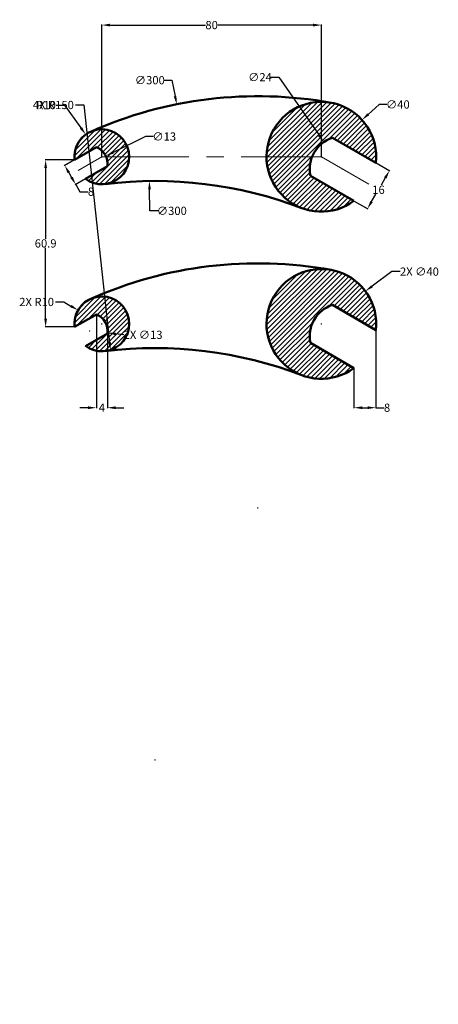
# Model space of a CAD drawing. Units: millimetres. Extents: x 67 to 219, y -177 to 182.
import ezdxf

# ---------------------------------------------------------------- set-up
doc = ezdxf.new("R2010")
doc.units = ezdxf.units.MM
doc.header["$MEASUREMENT"] = 0
doc.linetypes.add('CENTER', pattern=[50.8, 31.75, -6.35, 6.35, -6.35])
for name, color, linetype, lineweight in [('M-CNTR', 4, 'CENTER', 18), ('M-DIMS', 3, 'Continuous', 25), ('M-HATC', 8, 'Continuous', 18), ('M-OUTL', 7, 'Continuous', 50)]:
    doc.layers.add(name, color=color, linetype=linetype, lineweight=lineweight)
doc.styles.get("Standard").update_dxf_attribs({"font": 'arial.ttf'})
doc.dimstyles.get("Standard").update_dxf_attribs({"dimtxt": 3, "dimasz": 3, "dimexe": 0.18, "dimexo": 0.0625, "dimgap": 0.09, "dimtad": 0, "dimtih": 1, "dimtoh": 1, "dimdec": 1, "dimdsep": 46, "dimtxsty": 'Standard', "dimcen": 0.09, "dimadec": 0, "dimazin": 0, "dimtfac": 1, "dimtdec": 1, "dimtofl": 0, "dimtmove": 0, "dimatfit": 3, "dimfxl": 1, "dimtolj": 1, "dimtzin": 0, "dimarcsym": 0})

# ---------------------------------------------------------------- blocks, each defined once
blk = doc.blocks.new('*D1')
at = {"layer": 'Defpoints', "color": 0, "transparency": 16777216}
for p in [(86.84, 130.69), (90.84, 123.77), (87.25, 121.69)]:
    blk.add_point(p, dxfattribs=at)
at = {"layer": 'M-DIMS', "color": 0, "lineweight": -2, "transparency": 16777216}
for p, q in [((86.79, 130.66), (83.09, 128.53)), ((84.75, 126.02), (85.75, 124.29)), ((90.79, 123.73), (87.09, 121.6)), ((87.25, 121.69), (88.75, 119.09)), ((88.75, 119.09), (91.75, 119.09))]:
    blk.add_line(p, q, dxfattribs=at)
at = {"layer": 'M-DIMS', "color": 0, "transparency": 16777216}
for points in [[(85.18, 126.27), (84.31, 125.77), (83.25, 128.62)], [(86.18, 124.54), (85.31, 124.04), (87.25, 121.69)]]:
    blk.add_solid(points, dxfattribs=at)
at = {"layer": 'M-DIMS', "color": 0, "transparency": 16777216, "insert": (92.83, 119.09), "char_height": 3, "attachment_point": 5}
blk.add_mtext('\\A1;8', dxfattribs=at)
blk = doc.blocks.new('*D2')
at = {"layer": 'Defpoints', "color": 0, "transparency": 16777216}
for p in [(176.78, 179.79), (96.78, 131.81), (176.78, 131.81)]:
    blk.add_point(p, dxfattribs=at)
at = {"layer": 'M-DIMS', "color": 0, "lineweight": -2, "transparency": 16777216}
for p, q in [((96.78, 131.87), (96.78, 179.97)), ((99.78, 179.79), (134.55, 179.79)), ((173.78, 179.79), (139.02, 179.79)), ((176.78, 131.87), (176.78, 179.97))]:
    blk.add_line(p, q, dxfattribs=at)
at = {"layer": 'M-DIMS', "color": 0, "transparency": 16777216}
for points in [[(99.78, 180.29), (99.78, 179.29), (96.78, 179.79)], [(173.78, 180.29), (173.78, 179.29), (176.78, 179.79)]]:
    blk.add_solid(points, dxfattribs=at)
at = {"layer": 'M-DIMS', "color": 0, "transparency": 16777216, "insert": (136.78, 179.79), "char_height": 3, "attachment_point": 5}
blk.add_mtext('\\A1;80', dxfattribs=at)
blk = doc.blocks.new('*D3')
at = {"layer": 'Defpoints', "color": 0, "transparency": 16777216}
for p in [(98.19, 132.1), (86.5, 126.4)]:
    blk.add_point(p, dxfattribs=at)
at = {"layer": 'M-DIMS', "color": 0, "lineweight": -2, "transparency": 16777216}
for p, q in [((112.66, 139.18), (100.88, 133.42)), ((115.66, 139.18), (112.66, 139.18)), ((92.25, 129.25), (92.43, 129.25)), ((92.34, 129.16), (92.34, 129.34))]:
    blk.add_line(p, q, dxfattribs=at)
at = {"layer": 'M-DIMS', "color": 0, "transparency": 16777216}
blk.add_solid([(100.66, 133.87), (101.1, 132.97), (98.19, 132.1)], dxfattribs=at)
at = {"layer": 'M-DIMS', "color": 0, "transparency": 16777216, "insert": (119.53, 139.18), "char_height": 3, "attachment_point": 5}
blk.add_mtext('\\A1;∅13', dxfattribs=at)
blk = doc.blocks.new('*D4')
at = {"layer": 'Defpoints', "color": 0, "transparency": 16777216}
for p in [(114.11, 122.98), (118.2, -177)]:
    blk.add_point(p, dxfattribs=at)
at = {"layer": 'M-DIMS', "color": 0, "lineweight": -2, "transparency": 16777216}
for p, q in [((114.26, 112.11), (114.15, 119.98)), ((117.26, 112.11), (114.26, 112.11))]:
    blk.add_line(p, q, dxfattribs=at)
at = {"layer": 'M-DIMS', "color": 0, "transparency": 16777216}
blk.add_solid([(114.65, 119.98), (113.65, 119.97), (114.11, 122.98)], dxfattribs=at)
at = {"layer": 'M-DIMS', "color": 0, "transparency": 16777216, "insert": (122.29, 112.11), "char_height": 3, "attachment_point": 5}
blk.add_mtext('\\A1;∅300', dxfattribs=at)
blk = doc.blocks.new('*D5')
at = {"layer": 'Defpoints', "color": 0, "transparency": 16777216}
for p in [(177.68, 137.19), (191.38, 117.49)]:
    blk.add_point(p, dxfattribs=at)
at = {"layer": 'M-DIMS', "color": 0, "lineweight": -2, "transparency": 16777216}
for p, q in [((158.27, 160.81), (161.27, 160.81)), ((161.27, 160.81), (175.97, 139.66)), ((184.44, 127.34), (184.62, 127.34)), ((184.53, 127.25), (184.53, 127.43))]:
    blk.add_line(p, q, dxfattribs=at)
at = {"layer": 'M-DIMS', "color": 0, "transparency": 16777216}
blk.add_solid([(176.38, 139.94), (175.56, 139.37), (177.68, 137.19)], dxfattribs=at)
at = {"layer": 'M-DIMS', "color": 0, "transparency": 16777216, "insert": (154.41, 160.81), "char_height": 3, "attachment_point": 5}
blk.add_mtext('\\A1;∅24', dxfattribs=at)
blk = doc.blocks.new('*D6')
at = {"layer": 'Defpoints', "color": 0, "transparency": 16777216}
for p in [(191.6, 145.25), (161.96, 118.38)]:
    blk.add_point(p, dxfattribs=at)
at = {"layer": 'M-DIMS', "color": 0, "lineweight": -2, "transparency": 16777216}
for p, q in [((197.79, 150.86), (193.82, 147.26)), ((200.79, 150.86), (197.79, 150.86)), ((176.69, 131.81), (176.87, 131.81)), ((176.78, 131.72), (176.78, 131.9))]:
    blk.add_line(p, q, dxfattribs=at)
at = {"layer": 'M-DIMS', "color": 0, "transparency": 16777216}
blk.add_solid([(193.49, 147.63), (194.16, 146.89), (191.6, 145.25)], dxfattribs=at)
at = {"layer": 'M-DIMS', "color": 0, "transparency": 16777216, "insert": (204.66, 150.86), "char_height": 3, "attachment_point": 5}
blk.add_mtext('\\A1;∅40', dxfattribs=at)
blk = doc.blocks.new('*D7')
at = {"layer": 'Defpoints', "color": 0, "transparency": 16777216}
for p in [(90.91, 139.91), (96.78, 131.81)]:
    blk.add_point(p, dxfattribs=at)
at = {"layer": 'M-DIMS', "color": 0, "lineweight": -2, "transparency": 16777216}
for p, q in [((80.12, 150.64), (83.12, 150.64)), ((83.12, 150.64), (89.15, 142.33)), ((96.69, 131.81), (96.87, 131.81)), ((96.78, 131.72), (96.78, 131.9))]:
    blk.add_line(p, q, dxfattribs=at)
at = {"layer": 'M-DIMS', "color": 0, "transparency": 16777216}
blk.add_solid([(89.55, 142.63), (88.74, 142.04), (90.91, 139.91)], dxfattribs=at)
at = {"layer": 'M-DIMS', "color": 0, "transparency": 16777216, "insert": (76.45, 150.64), "char_height": 3, "attachment_point": 5}
blk.add_mtext('\\A1;R10', dxfattribs=at)
blk = doc.blocks.new('*D8')
at = {"layer": 'Defpoints', "color": 0, "transparency": 16777216}
for p in [(196.66, 129.58), (188.66, 115.72), (193.59, 112.87)]:
    blk.add_point(p, dxfattribs=at)
at = {"layer": 'M-DIMS', "color": 0, "lineweight": -2, "transparency": 16777216}
for p, q in [((196.71, 129.54), (201.74, 126.64)), ((200.09, 124.13), (198.52, 121.42)), ((188.71, 115.69), (193.74, 112.78)), ((195.09, 115.47), (196.65, 118.18))]:
    blk.add_line(p, q, dxfattribs=at)
at = {"layer": 'M-DIMS', "color": 0, "transparency": 16777216}
for points in [[(199.65, 124.38), (200.52, 123.88), (201.59, 126.73)], [(194.65, 115.72), (195.52, 115.22), (193.59, 112.87)]]:
    blk.add_solid(points, dxfattribs=at)
at = {"layer": 'M-DIMS', "color": 0, "transparency": 16777216, "insert": (197.59, 119.8), "char_height": 3, "attachment_point": 5}
blk.add_mtext('\\A1;16', dxfattribs=at)
blk = doc.blocks.new('*D9')
at = {"layer": 'Defpoints', "color": 0, "transparency": 16777216}
for p in [(124.06, 150.94), (183.25, -143.17)]:
    blk.add_point(p, dxfattribs=at)
at = {"layer": 'M-DIMS', "color": 0, "lineweight": -2, "transparency": 16777216}
for p, q in [((119.29, 159.72), (122.29, 159.72)), ((122.29, 159.72), (123.47, 153.88)), ((153.57, 3.89), (153.75, 3.89)), ((153.66, 3.8), (153.66, 3.98))]:
    blk.add_line(p, q, dxfattribs=at)
at = {"layer": 'M-DIMS', "color": 0, "transparency": 16777216}
blk.add_solid([(123.96, 153.98), (122.98, 153.78), (124.06, 150.94)], dxfattribs=at)
at = {"layer": 'M-DIMS', "color": 0, "transparency": 16777216, "insert": (114.26, 159.72), "char_height": 3, "attachment_point": 5}
blk.add_mtext('\\A1;∅300', dxfattribs=at)
blk = doc.blocks.new('SPANNER-DOUBLE-OPEN-8X16')
for p, q in [((94, 26.93), (109.87, 17.76)), ((8, 23.46), (0.06, 18.88)), ((12, 16.54), (4.06, 11.95)), ((86, 13.07), (101.87, 3.91))]:
    blk.add_line(p, q)
for centre, radius, start, end in [((66.87, -107.93), 150, 79.7534, 113.9695), ((90, 20), 20, 353.5782, 306.4218), ((10, 20), 10, 233.5782, 186.4218), ((97.75, 15.53), 12, 108.1897, 191.8103), ((5.56, 17.44), 6.5, 352.0201, 67.9799), ((29.37, -138.82), 150, 69.1074, 96.9552)]:
    blk.add_arc(centre, radius, start, end)
blk = doc.blocks.new('*D11')
at = {"layer": 'Defpoints', "color": 0, "transparency": 16777216}
for p in [(86.84, 130.69), (76.29, 69.79), (86.84, 69.79)]:
    blk.add_point(p, dxfattribs=at)
at = {"layer": 'M-DIMS', "color": 0, "lineweight": -2, "transparency": 16777216}
for p, q in [((86.78, 130.69), (76.11, 130.69)), ((76.29, 127.69), (76.29, 101.86)), ((76.29, 72.79), (76.29, 98.62)), ((86.78, 69.79), (76.11, 69.79))]:
    blk.add_line(p, q, dxfattribs=at)
at = {"layer": 'M-DIMS', "color": 0, "transparency": 16777216}
for points in [[(75.79, 127.69), (76.79, 127.69), (76.29, 130.69)], [(75.79, 72.79), (76.79, 72.79), (76.29, 69.79)]]:
    blk.add_solid(points, dxfattribs=at)
at = {"layer": 'M-DIMS', "color": 0, "transparency": 16777216, "insert": (76.29, 100.24), "char_height": 3, "attachment_point": 5}
blk.add_mtext('\\A1;60.9', dxfattribs=at)
blk = doc.blocks.new('*D12')
at = {"layer": 'Defpoints', "color": 0, "transparency": 16777216}
for p in [(94.781982, 74.372477), (98.781982, 67.444274), (98.781982, 40.38031)]:
    blk.add_point(p, dxfattribs=at)
at = {"layer": 'M-DIMS', "color": 0, "lineweight": -2, "transparency": 16777216}
for p, q in [((94.781982, 74.309977), (94.781982, 40.20031)), ((98.781982, 67.381774), (98.781982, 40.20031)), ((91.781982, 40.38031), (88.781982, 40.38031)), ((101.781982, 40.38031), (104.781982, 40.38031))]:
    blk.add_line(p, q, dxfattribs=at)
at = {"layer": 'M-DIMS', "color": 0, "transparency": 16777216}
for points in [[(91.781982, 40.88031), (91.781982, 39.88031), (94.781982, 40.38031)], [(101.781982, 40.88031), (101.781982, 39.88031), (98.781982, 40.38031)]]:
    blk.add_solid(points, dxfattribs=at)
at = {"layer": 'M-DIMS', "color": 0, "transparency": 16777216, "insert": (96.781982, 40.38031), "char_height": 3, "attachment_point": 5}
blk.add_mtext('\\A1;4', dxfattribs=at)
blk = doc.blocks.new('*D13')
at = {"layer": 'Defpoints', "color": 0, "transparency": 16777216}
for p in [(196.66, 68.67), (188.66, 54.82), (196.66, 40.38)]:
    blk.add_point(p, dxfattribs=at)
at = {"layer": 'M-DIMS', "color": 0, "lineweight": -2, "transparency": 16777216}
for p, q in [((196.66, 68.61), (196.66, 40.2)), ((188.66, 54.75), (188.66, 40.2)), ((191.66, 40.38), (193.66, 40.38)), ((196.66, 40.38), (199.66, 40.38))]:
    blk.add_line(p, q, dxfattribs=at)
at = {"layer": 'M-DIMS', "color": 0, "transparency": 16777216}
for points in [[(191.66, 40.88), (191.66, 39.88), (188.66, 40.38)], [(193.66, 40.88), (193.66, 39.88), (196.66, 40.38)]]:
    blk.add_solid(points, dxfattribs=at)
at = {"layer": 'M-DIMS', "color": 0, "transparency": 16777216, "insert": (200.73, 40.38), "char_height": 3, "attachment_point": 5}
blk.add_mtext('\\A1;8', dxfattribs=at)
blk = doc.blocks.new('*D14')
at = {"layer": 'Defpoints', "color": 0, "transparency": 16777216}
for p in [(192.85, 82.82), (160.72, 58.99)]:
    blk.add_point(p, dxfattribs=at)
at = {"layer": 'M-DIMS', "color": 0, "lineweight": -2, "transparency": 16777216}
for p, q in [((202.48, 89.97), (195.25, 84.61)), ((205.48, 89.97), (202.48, 89.97)), ((176.69, 70.91), (176.87, 70.91)), ((176.78, 70.82), (176.78, 71))]:
    blk.add_line(p, q, dxfattribs=at)
at = {"layer": 'M-DIMS', "color": 0, "transparency": 16777216}
blk.add_solid([(194.96, 85.01), (195.55, 84.21), (192.85, 82.82)], dxfattribs=at)
at = {"layer": 'M-DIMS', "color": 0, "transparency": 16777216, "insert": (212.52, 89.97), "char_height": 3, "attachment_point": 5}
blk.add_mtext('\\A1;2X ∅40', dxfattribs=at)
blk = doc.blocks.new('*D15')
at = {"layer": 'Defpoints', "color": 0, "transparency": 16777216}
for p in [(88.12, 75.91), (96.78, 70.91)]:
    blk.add_point(p, dxfattribs=at)
at = {"layer": 'M-DIMS', "color": 0, "lineweight": -2, "transparency": 16777216}
for p, q in [((79.93, 78.91), (82.93, 78.91)), ((82.93, 78.91), (85.52, 77.41)), ((96.69, 70.91), (96.87, 70.91)), ((96.78, 70.82), (96.78, 71))]:
    blk.add_line(p, q, dxfattribs=at)
at = {"layer": 'M-DIMS', "color": 0, "transparency": 16777216}
blk.add_solid([(85.77, 77.84), (85.27, 76.98), (88.12, 75.91)], dxfattribs=at)
at = {"layer": 'M-DIMS', "color": 0, "transparency": 16777216, "insert": (73.01, 78.91), "char_height": 3, "attachment_point": 5}
blk.add_mtext('\\A1;2X R10', dxfattribs=at)
blk = doc.blocks.new('*D16')
at = {"layer": 'Defpoints', "color": 0, "transparency": 16777216}
for p in [(85.89, 69.08), (98.8, 67.62)]:
    blk.add_point(p, dxfattribs=at)
at = {"layer": 'M-DIMS', "color": 0, "lineweight": -2, "transparency": 16777216}
for p, q in [((92.25, 68.35), (92.43, 68.35)), ((92.34, 68.26), (92.34, 68.44)), ((104.77, 66.94), (101.78, 67.28))]:
    blk.add_line(p, q, dxfattribs=at)
at = {"layer": 'M-DIMS', "color": 0, "transparency": 16777216}
blk.add_solid([(101.84, 67.78), (101.73, 66.78), (98.8, 67.62)], dxfattribs=at)
at = {"layer": 'M-DIMS', "color": 0, "transparency": 16777216, "insert": (111.81, 66.94), "char_height": 3, "attachment_point": 5}
blk.add_mtext('\\A1;2X ∅13', dxfattribs=at)
blk = doc.blocks.new('*D17')
at = {"layer": 'Defpoints', "color": 0, "transparency": 16777216}
for p in [(99.95, 61.21), (116.16, -87.91)]:
    blk.add_point(p, dxfattribs=at)
at = {"layer": 'M-DIMS', "color": 0, "lineweight": -2, "transparency": 16777216}
for p, q in [((87.22, 150.68), (90.22, 150.68)), ((90.22, 150.68), (99.62, 64.19)), ((116.07, -87.91), (116.25, -87.91)), ((116.16, -88), (116.16, -87.82))]:
    blk.add_line(p, q, dxfattribs=at)
at = {"layer": 'M-DIMS', "color": 0, "transparency": 16777216}
blk.add_solid([(100.12, 64.24), (99.13, 64.14), (99.95, 61.21)], dxfattribs=at)
at = {"layer": 'M-DIMS', "color": 0, "transparency": 16777216, "insert": (79.1, 150.68), "char_height": 3, "attachment_point": 5}
blk.add_mtext('\\A1;4X R150', dxfattribs=at)

msp = doc.modelspace()

# ---------------------------------------------------------------- hatches: boundary and pattern name
at = {"layer": 'M-HATC'}
h = msp.add_hatch(dxfattribs=at)
h.set_pattern_fill('ANSI31', color=256, scale=10)
h.set_pattern_definition([(45, (81.8162, 116.579), (-0.883883, 0.883883), [])])
h.paths.add_polyline_path([(86.84, 130.69), (94.78, 135.28, -0.197866), (98.32, 131.81), (106.78, 131.81, 1.057672)])
h.paths.add_polyline_path([(106.78, 131.81), (98.32, 131.81, -0.136941), (98.78, 128.35), (90.84, 123.77, 0.615335)])
h.paths.add_polyline_path([(172.78, 124.88, -0.148074), (173.39, 131.81), (156.78, 131.81, 0.615335), (188.66, 115.72)])
h.paths.add_polyline_path([(180.78, 138.74), (196.66, 129.58, 1.057672), (156.78, 131.81), (173.39, 131.81, -0.221372)])
h = msp.add_hatch(dxfattribs=at)
h.set_pattern_fill('ANSI31', color=256, scale=10)
h.set_pattern_definition([(45, (81.8162, 55.6749), (-0.883883, 0.883883), [])])
h.paths.add_polyline_path([(86.84, 69.79), (94.78, 74.37, -0.197866), (98.32, 70.91), (106.78, 70.91, 1.057672)])
h.paths.add_polyline_path([(106.78, 70.91), (98.32, 70.91, -0.136941), (98.78, 67.44), (90.84, 62.86, 0.615335)])
h.paths.add_polyline_path([(172.78, 63.98, -0.148074), (173.39, 70.91), (156.78, 70.91, 0.615335), (188.66, 54.82)])
h.paths.add_polyline_path([(180.78, 77.84), (196.66, 68.67, 1.057672), (156.78, 70.91), (173.39, 70.91, -0.221372)])

# ---------------------------------------------------------------- linework, layer by layer
at = {"layer": 'M-CNTR'}
for p, q in [((96.78, 131.81), (88.12, 126.81)), ((96.78, 131.81), (176.78, 131.81)), ((176.78, 131.81), (194.1, 121.81))]:
    msp.add_line(p, q, dxfattribs=at)

# ---------------------------------------------------------------- block references
at = {"layer": 'M-OUTL'}
for p in [(86.78, 111.81), (86.78, 50.91)]:
    msp.add_blockref('SPANNER-DOUBLE-OPEN-8X16', p, dxfattribs=at)

# ---------------------------------------------------------------- dimensions: what is measured, and where the dimension line sits
at = {"layer": 'M-DIMS', "transparency": 33554610}
dim = msp.add_linear_dim(base=(176.78, 179.79), p1=(96.78, 131.81), p2=(176.78, 131.81), dimstyle='Standard', override={"dimclrd": 0, "dimclre": 0, "dimclrt": 0}, dxfattribs=at)
dim.commit()
dim.dimension.update_dxf_attribs({"geometry": '*D2', "text_midpoint": (136.78, 179.79)})
for p1, p2, picture, middle in [((183.25, -143.17), (124.06, 150.94), '*D9', (114.26, 159.72)), ((191.38, 117.49), (177.68, 137.19), '*D5', (154.41, 160.81)), ((161.96, 118.38), (191.6, 145.25), '*D6', (204.66, 150.86)), ((86.5, 126.4), (98.19, 132.1), '*D3', (119.53, 139.18)), ((118.2, -177), (114.11, 122.98), '*D4', (122.29, 112.11))]:
    dim = msp.add_diameter_dim_2p(p1=p1, p2=p2, dimstyle='Standard', override={"dimclrd": 0, "dimclre": 0, "dimclrt": 0}, dxfattribs=at)
    dim.commit()
    dim.dimension.update_dxf_attribs({"geometry": picture, "text_midpoint": middle, "dimtype": 163})
at = {"layer": 'M-DIMS'}
for center, mpoint, text, picture, middle in [((116.16, -87.91), (99.95, 61.21), '4X <>', '*D17', (79.1, 150.68)), ((96.78, 70.91), (88.12, 75.91), '2X <>', '*D15', (73.01, 78.91))]:
    dim = msp.add_radius_dim(center=center, mpoint=mpoint, text=text, dimstyle='Standard', override={"dimdec": 0, "dimlfac": 1, "dimrnd": 0, "dimzin": 0, "dimdsep": 46, "dimlunit": 2}, dxfattribs=at)
    dim.commit()
    dim.dimension.update_dxf_attribs({"geometry": picture, "text_midpoint": middle, "dimtype": 164})
at = {"layer": 'M-DIMS', "transparency": 33554610}
dim = msp.add_radius_dim(center=(96.78, 131.81), mpoint=(90.91, 139.91), dimstyle='Standard', override={"dimclrd": 0, "dimclre": 0, "dimclrt": 0}, dxfattribs=at)
dim.commit()
dim.dimension.update_dxf_attribs({"geometry": '*D7', "text_midpoint": (76.45, 150.64), "dimtype": 164})
at = {"layer": 'M-DIMS'}
dim = msp.add_linear_dim(base=(76.29, 69.79), p1=(86.84, 130.69), p2=(86.84, 69.79), angle=90, dimstyle='Standard', override={"dimdec": 1, "dimlfac": 1, "dimrnd": 0, "dimzin": 0, "dimdsep": 46, "dimlunit": 2}, dxfattribs=at)
dim.commit()
dim.dimension.update_dxf_attribs({"geometry": '*D11', "text_midpoint": (76.29, 100.24)})
at = {"layer": 'M-DIMS', "transparency": 33554610}
for p1, p2, distance, picture, middle in [((86.84, 130.69), (90.84, 123.77), -4.15, '*D1', (92.83, 119.09)), ((196.66, 129.58), (188.66, 115.72), 5.69, '*D8', (197.59, 119.8))]:
    dim = msp.add_aligned_dim(p1=p1, p2=p2, distance=distance, dimstyle='Standard', override={"dimclrd": 0, "dimclre": 0, "dimclrt": 0}, dxfattribs=at)
    dim.commit()
    dim.dimension.update_dxf_attribs({"geometry": picture, "text_midpoint": middle})
at = {"layer": 'M-DIMS'}
for p1, p2, picture, middle in [((160.72, 58.99), (192.85, 82.82), '*D14', (212.52, 89.97)), ((85.89, 69.08), (98.8, 67.62), '*D16', (104.77, 66.94))]:
    dim = msp.add_diameter_dim_2p(p1=p1, p2=p2, text='2X <>', dimstyle='Standard', override={"dimdec": 0, "dimlfac": 1, "dimrnd": 0, "dimzin": 0, "dimdsep": 46, "dimlunit": 2}, dxfattribs=at)
    dim.commit()
    dim.dimension.update_dxf_attribs({"geometry": picture, "text_midpoint": middle, "dimtype": 163})
for base, p1, p2, picture, middle in [((98.78, 40.38), (94.78, 74.37), (98.78, 67.44), '*D12', (96.78, 40.38)), ((196.66, 40.38), (188.66, 54.82), (196.66, 68.67), '*D13', (200.73, 40.38))]:
    dim = msp.add_linear_dim(base=base, p1=p1, p2=p2, dimstyle='Standard', override={"dimdec": 0, "dimlfac": 1, "dimrnd": 0, "dimzin": 0, "dimdsep": 46, "dimlunit": 2}, dxfattribs=at)
    dim.commit()
    dim.dimension.update_dxf_attribs({"geometry": picture, "text_midpoint": middle})

doc.saveas('drawing.dxf')
